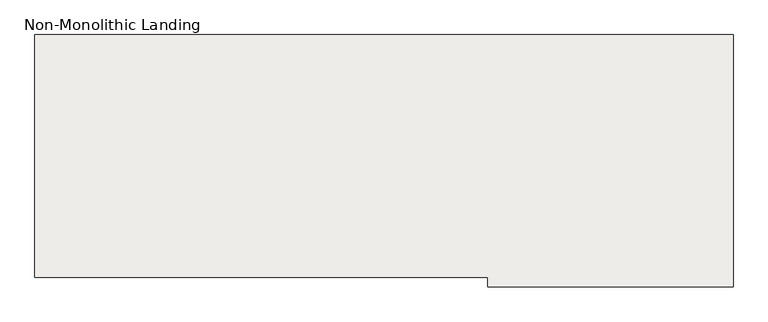
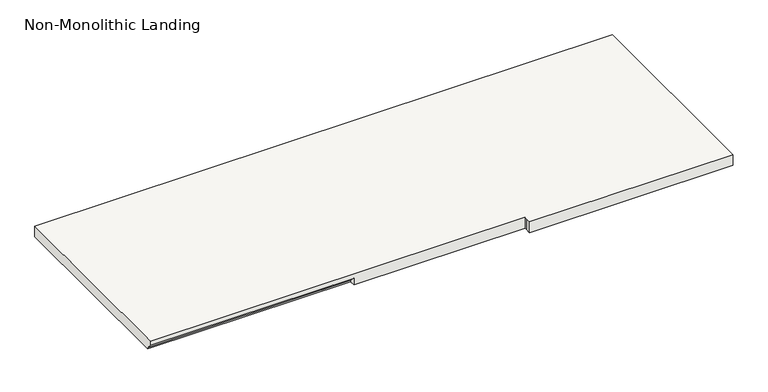
"""IFC4 building model written with IfcOpenShell, lengths in millimetres: slab geometry, Non-Monolithic Landing."""

from ifc_helpers import new_model, si_unit, origin, place, context, project, spatial, faceted_brep, source, transform, mapped, element, save


def non_monolithic_landing_a2679692(model_context):
    return source(origin(), model_context, "Body", "Brep", [
        faceted_brep([(-7448.5867944, 13309.8230289, 1581.15), (-7448.5867944, 13335.2230289, 1555.75), (-6534.1867944, 13335.2230289, 1555.75), (-6534.1867944, 13309.8230289, 1581.15), (-5762.1737939, 13309.8230289, 1600.2), (-5762.1737939, 13300.0419954, 1600.2), (-5762.1737939, 13274.6419954, 1600.2), (-4847.7737939, 13274.6419954, 1600.2), (-4847.7737939, 13300.0419954, 1600.2), (-4847.7737939, 14214.4419954, 1600.2), (-7448.5867944, 14214.4419954, 1600.2), (-7448.5867944, 13309.8230289, 1600.2), (-6534.1867944, 13335.2230289, 1549.4), (-7448.5867944, 13335.2230289, 1549.4), (-7448.5867944, 14214.4419954, 1549.4), (-4847.7737939, 14214.4419954, 1549.4), (-4847.7737939, 13300.0419954, 1549.4), (-4847.7737939, 13274.6419954, 1549.4), (-5762.1737939, 13274.6419954, 1549.4), (-5762.1737939, 13300.0419954, 1549.4), (-5762.1737939, 13309.8230289, 1549.4), (-6534.1867944, 13309.8230289, 1549.4)], [[[0, 1, 2, 3]], [[4, 5, 6, 7, 8, 9, 10, 11]], [[12, 13, 14, 15, 16, 17, 18, 19, 20, 21]], [[13, 12, 2, 1]], [[4, 11, 0, 3, 21, 20]], [[5, 4, 20, 19]], [[6, 5, 19, 18]], [[7, 6, 18, 17]], [[8, 7, 17, 16]], [[9, 8, 16, 15]], [[10, 9, 15, 14]], [[11, 10, 14, 13, 1, 0]], [[12, 21, 3, 2]]]),
    ])


if __name__ == "__main__":
    model = new_model("IFC4")
    model_context = context("Model", 3, world=origin())
    ifc_project = project(units=[si_unit("LENGTHUNIT", "METRE", prefix="MILLI")], contexts=[model_context])
    site = spatial("IfcSite", under=ifc_project)
    building = spatial("IfcBuilding", under=site)
    placement = place(None, origin())
    non_monolithic_landing_shape = non_monolithic_landing_a2679692(model_context)
    element("IfcSlab", 1, ObjectType="Non-Monolithic Landing", at=placement, inside=building, context=model_context, shape_type="MappedRepresentation", body=[
        mapped(non_monolithic_landing_shape, transform((0.0, 0.0, 0.0), x_axis=(1.0, 0.0, 0.0), y_axis=(0.0, 1.0, 0.0), z_axis=(0.0, 0.0, 1.0))),
    ])
    save(model, "model.ifc")
